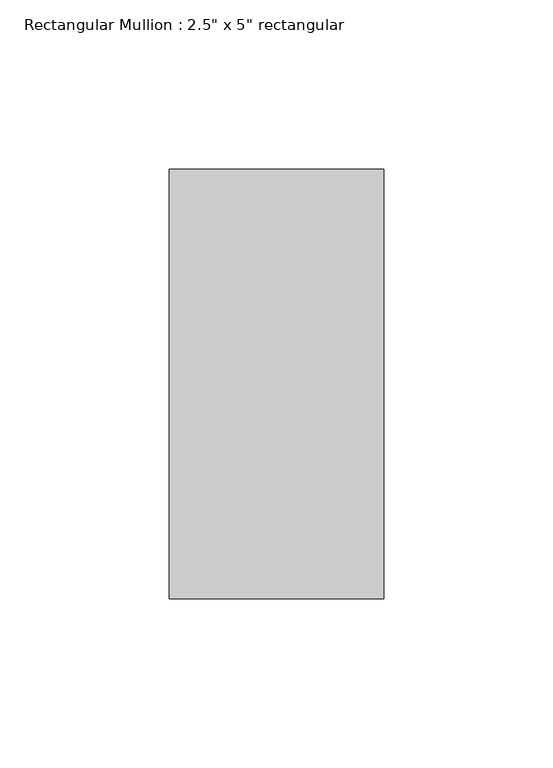
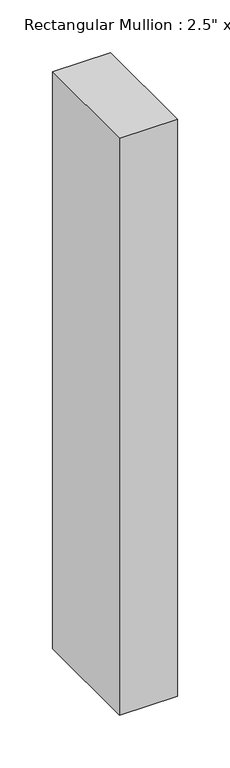
"""IFC4 building model written with IfcOpenShell, lengths in millimetres: member geometry."""

from ifc_helpers import new_model, si_unit, frame, origin, place, context, project, spatial, polyline, outline, extrude, source, transform, mapped, element, save


def member_d41206f4(model_context):
    return source(origin(), model_context, "Body", "SweptSolid", [
        extrude(outline(polyline([(0.0, 63.5), (0.0, -63.5), (-63.5, -63.5), (-63.5, 63.5), (0.0, 63.5)])), frame((0.0, 0.0, -668.3375), z_axis=(0.0, 0.0, 1.0), x_axis=(1.0, 0.0, 0.0)), (0.0, 0.0, 1.0), 668.3375),
    ])


if __name__ == "__main__":
    model = new_model("IFC4")
    model_context = context("Model", 3, world=origin())
    ifc_project = project(units=[si_unit("LENGTHUNIT", "METRE", prefix="MILLI")], contexts=[model_context])
    site = spatial("IfcSite", under=ifc_project)
    building = spatial("IfcBuilding", under=site)
    placement = place(None, origin())
    member_shape = member_d41206f4(model_context)
    element("IfcMember", 1, ObjectType="Rectangular Mullion : 2.5\" x 5\" rectangular", at=placement, inside=building, context=model_context, shape_type="MappedRepresentation", body=[
        mapped(member_shape, transform((0.0, 0.0, 0.0), x_axis=(1.0, 0.0, 0.0), y_axis=(0.0, 1.0, 0.0), z_axis=(0.0, 0.0, 1.0))),
    ])
    save(model, "model.ifc")

# Revit data of these elements
# Type "Rectangular Mullion : 2.5\" x 5\" rectangular"
#   built-in parameter 1007304 = 0.416667 (stored number, unit not read)
#   built-in parameter 1007301 = 0.104167 (stored number, unit not read)
#   built-in parameter 1007300 = 0.104167 (stored number, unit not read)
# Element 1 (IfcMember, "Rectangular Mullion : 2.5\" x 5\" rectangular")
#   Materials on its faces: "Aluminum"
# Materials
#   "Aluminum": class "Metal", colour RGB 247 247 247, transparency 0, Description = "Aluminum 6061", Cost = 0
